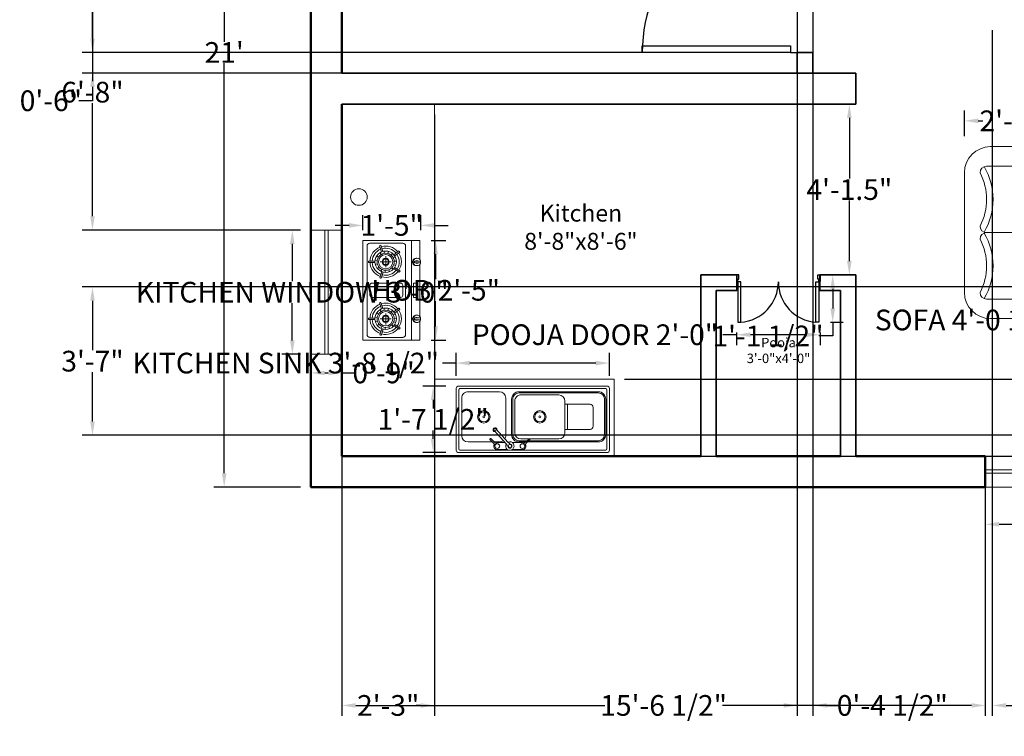
# Model space of a CAD drawing. Units: inches. Extents: x -59 to 502, y -260 to 136.
# Tile 1 of 8: x -59 to 226, y -260 to -53. Entities that reach past the tile are written whole.
import ezdxf

# ---------------------------------------------------------------- set-up
doc = ezdxf.new("R2010")
doc.units = ezdxf.units.IN
doc.header["$MEASUREMENT"] = 0
for name, color, linetype, lineweight in [('A-ANNO-DIMS', 2, 'Continuous', 18), ('A-AREA-IDEN', 7, 'Continuous', 25), ('A-FLOR-CASE', 9, 'Continuous', 18), ('Doors', 18, 'Continuous', 25), ('Inner wall', 11, 'Continuous', 35), ('Kitchen Appliances', 80, 'Continuous', 18), ('Outer Wall', 10, 'Continuous', 50), ('Sink', 62, 'Continuous', 18), ('Sofas', 84, 'Continuous', 18), ('Windows', 150, 'Continuous', 18)]:
    doc.layers.add(name, color=color, linetype=linetype, lineweight=lineweight)
doc.styles.get("Standard").update_dxf_attribs({"font": 'arial.ttf'})
doc.dimstyles.get("Standard").update_dxf_attribs({"dimtxt": 6, "dimasz": 4, "dimexe": 3, "dimexo": 3, "dimgap": 0.09, "dimtad": 0, "dimtih": 1, "dimtoh": 1, "dimdec": 1, "dimzin": 0, "dimdsep": 46, "dimlunit": 3, "dimtxsty": 'Standard', "dimcen": 0.09, "dimadec": 0, "dimazin": 0, "dimtfac": 1, "dimtdec": 1, "dimtofl": 0, "dimtmove": 0, "dimatfit": 3, "dimfxl": 1, "dimtolj": 1, "dimtzin": 0, "dimarcsym": 0})

# ---------------------------------------------------------------- blocks, each defined once
blk = doc.blocks.new('Window')
for p, q in [((868.39, 234.72), (940.39, 234.72)), ((868.39, 225.72), (868.39, 234.72)), ((940.39, 234.72), (940.39, 225.72)), ((868.39, 230.72), (940.39, 230.72)), ((940.39, 229.72), (868.39, 229.72)), ((940.39, 225.72), (868.39, 225.72))]:
    blk.add_line(p, q)
blk = doc.blocks.new('*D6')
at = {"layer": 'A-ANNO-DIMS', "color": 0, "lineweight": -2, "transparency": 16777216}
for p, q in [((22.46, 63.92), (-2.69, 63.92)), ((0.31, 59.92), (0.31, -58.98)), ((0.31, -184.08), (0.31, -65.18)), ((22.46, -188.08), (-2.69, -188.08))]:
    blk.add_line(p, q, dxfattribs=at)
at = {"layer": 'A-ANNO-DIMS', "color": 0, "transparency": 16777216}
for points in [[(-0.35, 59.92), (0.98, 59.92), (0.31, 63.92)], [(-0.35, -184.08), (0.98, -184.08), (0.31, -188.08)]]:
    blk.add_solid(points, dxfattribs=at)
at = {"layer": 'Defpoints', "color": 0, "transparency": 16777216}
for p in [(25.46, 63.92), (0.31, -188.08), (25.46, -188.08)]:
    blk.add_point(p, dxfattribs=at)
at = {"layer": 'A-ANNO-DIMS', "color": 0, "transparency": 16777216, "insert": (0.31, -62.08), "char_height": 6, "attachment_point": 5}
blk.add_mtext("\\A1;21'", dxfattribs=at)
blk = doc.blocks.new('*U11')
for p, q in [((-40, 0), (-40, 6)), ((0, 0), (0, 6))]:
    blk.add_line(p, q)
blk.add_lwpolyline([(0, 0), (0, -40), (-1.75, -40), (-1.75, 0)], close=True)
blk.add_arc((0, 0), 40, 180, 270)
blk = doc.blocks.new('Kitchen Window KW')
for p, q in [((875.78, 183.9), (911.78, 183.9)), ((875.78, 174.9), (875.78, 183.9)), ((911.78, 183.9), (911.78, 174.9)), ((875.78, 179.9), (911.78, 179.9)), ((911.78, 178.9), (875.78, 178.9)), ((911.78, 174.9), (875.78, 174.9))]:
    blk.add_line(p, q)
blk = doc.blocks.new('A$C16D51D41')
for p, q in [((1.12, 0.69, -343.199), (0.2, 0.69, -343.199)), ((0, 0.49, -343.199), (0, 0.06, -343.199)), ((0.15, 0.52, -343.199), (0.15, 0.06, -343.199)), ((0.15, 0.06, -343.199), (0.15, 0.52, -343.199)), ((0.15, 0.52, -343.199), (0.15, 0.06, -343.199)), ((0.66, 0.06, -343.199), (0.66, 0.52, -343.199)), ((0.66, 0.52, -343.199), (0.66, 0.06, -343.199)), ((1.17, 0.52, -343.199), (1.17, 0.06, -343.199)), ((1.32, 0.06, -343.199), (1.32, 0.49, -343.199)), ((0, 0.06, -343.199), (0.15, 0.06, -343.199)), ((1.32, 0.06, -343.199), (1.17, 0.06, -343.199))]:
    blk.add_line(p, q)
for centre, radius, start, end in [((0.2, 0.49, -343.199), 0.2, 90, 180), ((1.12, 0.49, -343.199), 0.2, 0, 90), ((0.2, 0.52, -343.199), 0.05, 90, 180), ((0.405, 0.9652, -343.199), 0.4953, 239.49109, 300.50891), ((0.405, 0.9652, -343.199), 0.4453, 242.58608, 297.41392), ((0.61, 0.52, -343.199), 0.05, 0, 90), ((0.71, 0.52, -343.199), 0.05, 90, 180), ((0.915, 0.9652, -343.199), 0.4953, 239.49109, 300.50891), ((0.915, 0.9652, -343.199), 0.4453, 242.58608, 297.41392), ((1.12, 0.52, -343.199), 0.05, 0, 90), ((0.405, 0.5719, -343.199), 0.5719, 243.51896, 296.48104), ((0.915, 0.5719, -343.199), 0.5719, 243.51896, 296.48104)]:
    blk.add_arc(centre, radius, start, end)
blk = doc.blocks.new('A$C5D256BD7')
for points in [[(60, 678), (60, 100), (20, 100), (20, 678)], [(1140, 678), (1140, 100), (1180, 100), (1180, 678)], [(6, 10), (0, 10), (0, 90), (6, 90)], [(6, 100), (20, 100), (20, 60), (32, 60), (32, 16), (32, 0), (6, 0)], [(1194, 100), (1180, 100), (1180, 60), (1168, 60), (1168, 16), (1168, 0), (1194, 0)], [(1194, 10), (1200, 10), (1200, 90), (1194, 90)]]:
    blk.add_lwpolyline(points, close=True)
for centre, start, end in [((21, 100), 359.9362, 86.0902), ((1179, 100), 93.9098, 180.0638)]:
    blk.add_arc(centre, 579, start, end)
blk = doc.blocks.new('Kitchen Sink Set')
at = {"color": 0}
for p, q in [((1319.2, 504.5), (1319.2, 30.2)), ((2480.8, 523.9), (1338.6, 523.9)), ((1338.6, 494.8), (1338.6, 39.9)), ((2078, 504.5), (1348.2, 504.5)), ((2068.2, 500.1), (1989.5, 500.1)), ((2471.1, 504.5), (2094.7, 504.5)), ((2183.1, 500.1), (2104.5, 500.1)), ((2112.8, 458.4), (2208, 354)), ((2480.8, 39.9), (2480.8, 494.8)), ((2500.2, 504.5), (2500.2, 30.2)), ((1347.4, 383.5), (1347.4, 112.5)), ((1356.3, 383.5), (1356.3, 112.5)), ((1950.6, 441.6), (1405.5, 441.6)), ((1941.6, 432.7), (1405.5, 432.7)), ((1710.4, 417.4), (1933.2, 417.4)), ((1957.7, 448.5), (1934.5, 425.7)), ((1940.2, 417.4), (2000.8, 417.4)), ((1964.5, 441.6), (1941.3, 418.8)), ((2015.4, 432.7), (1955.4, 432.7)), ((2015.4, 441.6), (1964.4, 441.6)), ((2068.2, 446), (1989.5, 446)), ((2063.8, 112.5), (2063.8, 383.5)), ((2073.4, 112.5), (2073.4, 383.5)), ((2098.5, 445.3), (2193.7, 340.9)), ((2117.8, 102.8), (2117.8, 393.2)), ((2183.1, 446), (2124.1, 446)), ((2166.2, 441.6), (2207.3, 441.6)), ((2207.7, 441.2), (2230.5, 418)), ((2214.6, 448), (2237.4, 424.8)), ((2220.8, 441.6), (2408.2, 441.6)), ((2456.6, 102.8), (2456.6, 393.2)), ((1444.2, 320.6), (1444.2, 175.4)), ((1662, 344.8), (1468.4, 344.8)), ((1642.7, 151.2), (1642.7, 344.8)), ((1662, 127), (1662, 369)), ((2049.2, 127), (2049.2, 369)), ((1662, 151.2), (1468.4, 151.2)), ((1710.4, 78.6), (2000.8, 78.6)), ((1338.6, 10.8), (2480.8, 10.8)), ((1348.2, 30.2), (2471.1, 30.2)), ((1405.5, 64.1), (2015.4, 64.1)), ((1405.5, 54.4), (2015.4, 54.4)), ((2166.2, 54.4), (2408.2, 54.4))]:
    blk.add_line(p, q, dxfattribs=at)
for centre, radius in [((1989.5, 473), 18.1), ((2086.3, 473), 12.4), ((2183.1, 473), 18.1), ((2201.5, 346.7), 9.73), ((1855.6, 248), 48.4), ((1855.6, 248), 38.7), ((1855.6, 248), 8.23), ((2287.2, 248), 48.4), ((2287.2, 248), 38.7), ((2287.2, 248), 8.23)]:
    blk.add_circle(centre, radius, dxfattribs=at)
for centre, radius, start, end in [((1338.6, 504.5), 19.4, 90, 180), ((1348.2, 494.8), 9.68, 90, 180), ((1923.8, 483.1), 48.4, 314.49562, 351.33895), ((1989.5, 473), 27, 90, 209.88157), ((2086.3, 473), 32.5, 329.64442, 295.0423), ((2086.3, 473), 16.4, 16.07549, 248.61123), ((2062.7, 412.7), 48.4, 42.34336, 68.61123), ((2148.6, 491), 48.4, 196.07549, 222.34336), ((2183.1, 473), 27, 329.10967, 90), ((2249.1, 481.9), 48.4, 187.65229, 224.49562), ((2471.1, 494.8), 9.68, 0, 90), ((2480.8, 504.5), 19.4, 0, 90), ((1405.5, 383.5), 58.1, 90, 180), ((1405.5, 383.5), 49.2, 90, 180), ((1710.4, 369), 48.4, 90, 180), ((1710.4, 369), 48.4, 90, 91.14555), ((1936.7, 421.1), 5.11, 115.72387, 333.26737), ((1998.4, 407.1), 48.4, 97.65229, 134.49562), ((1989.5, 473), 27, 239.10967, 270), ((2000.8, 369), 48.4, 0, 90), ((2015.4, 383.5), 58.1, 0, 90), ((2013.9, 382.9), 49.8, 0.67291, 88.37528), ((2166.2, 393.2), 48.4, 150.29154, 180), ((2166.2, 393.2), 48.4, 90, 127.0737), ((2173.1, 407.3), 48.4, 44.49562, 81.33895), ((2183.1, 473), 27, 270, 299.88157), ((2235.1, 420.2), 5.11, 205.72387, 63.26737), ((2408.2, 393.2), 48.4, 0, 90), ((1468.4, 320.6), 24.2, 90, 180), ((2200.8, 347.4), 15.7, 170.3658, 94.32092), ((1468.4, 175.4), 24.2, 180, 270), ((1405.5, 112.5), 58.1, 180, 270), ((1406.1, 113.9), 49.8, 181.62472, 269.32709), ((1710.4, 127), 48.4, 180, 270), ((2000.8, 127), 48.4, 270, 0), ((2015.4, 112.5), 58.1, 270, 0), ((2015.4, 112.5), 48.4, 270, 0), ((2166.2, 102.8), 48.4, 180, 270), ((2408.2, 102.8), 48.4, 270, 0), ((1338.6, 30.2), 19.4, 180, 270), ((1348.2, 39.9), 9.68, 180, 270), ((2471.1, 39.9), 9.68, 270, 0), ((2480.8, 30.2), 19.4, 270, 0)]:
    blk.add_arc(centre, radius, start, end, dxfattribs=at)
blk = doc.blocks.new('Gas Stove')
for p, q in [((1373.89, 868.55), (1373.89, 856.72)), ((1373.89, 868.55), (1394.6, 868.55)), ((1375.08, 867.67), (1393.41, 867.67)), ((1394.6, 868.55), (1394.6, 856.72)), ((1374.48, 867.08), (1374.48, 860.27)), ((1377.75, 865.97), (1377.87, 865.54)), ((1378.18, 866.04), (1378.18, 867.37)), ((1378.48, 866.04), (1378.48, 867.37)), ((1378.68, 866.01), (1378.61, 865.58)), ((1379.54, 865.68), (1379.3, 865.31)), ((1382.77, 866.63), (1382.77, 860.72)), ((1383.21, 867.08), (1385.28, 867.08)), ((1385.72, 866.63), (1385.72, 860.72)), ((1389.59, 865.97), (1389.7, 865.54)), ((1390.01, 866.04), (1390.01, 867.37)), ((1390.31, 866.04), (1390.31, 867.37)), ((1390.51, 866.01), (1390.44, 865.58)), ((1391.37, 865.68), (1391.13, 865.31)), ((1394, 867.08), (1394, 860.27)), ((1374.9, 864.75), (1376.17, 864.35)), ((1374.99, 865.03), (1376.26, 864.63)), ((1376.11, 863.94), (1376.56, 863.92)), ((1376.35, 864.83), (1376.75, 864.63)), ((1376.93, 865.55), (1377.21, 865.2)), ((1377.16, 863.82), (1379.45, 863.82)), ((1378.33, 864.99), (1378.33, 862.65)), ((1380.19, 865.03), (1379.82, 864.79)), ((1380.52, 864.17), (1380.08, 864.1)), ((1381.65, 865.09), (1380.38, 864.66)), ((1381.74, 864.81), (1380.48, 864.38)), ((1386.73, 864.75), (1388, 864.35)), ((1386.82, 865.03), (1388.09, 864.63)), ((1387.94, 863.94), (1388.39, 863.92)), ((1388.18, 864.83), (1388.58, 864.63)), ((1388.76, 865.55), (1389.04, 865.2)), ((1389.01, 863.82), (1391.31, 863.82)), ((1390.16, 864.99), (1390.16, 862.65)), ((1392.02, 865.03), (1391.65, 864.79)), ((1392.35, 864.17), (1391.91, 864.1)), ((1393.48, 865.09), (1392.21, 864.66)), ((1393.57, 864.81), (1392.31, 864.38)), ((1376.15, 861.02), (1376.92, 862.11)), ((1376.26, 863.03), (1376.67, 863.19)), ((1376.39, 860.85), (1377.16, 861.94)), ((1376.76, 862.25), (1377.07, 862.57)), ((1377.53, 861.75), (1377.69, 862.17)), ((1378.44, 861.61), (1378.42, 862.05)), ((1379.34, 861.85), (1379.13, 862.24)), ((1380.32, 860.88), (1379.53, 861.95)), ((1380.05, 862.43), (1379.71, 862.71)), ((1380.56, 861.06), (1379.76, 862.13)), ((1380.47, 863.25), (1380.04, 863.36)), ((1387.98, 861.02), (1388.75, 862.11)), ((1388.09, 863.03), (1388.5, 863.19)), ((1388.22, 860.85), (1388.99, 861.94)), ((1388.59, 862.25), (1388.9, 862.57)), ((1389.36, 861.75), (1389.52, 862.17)), ((1390.28, 861.61), (1390.25, 862.05)), ((1391.17, 861.85), (1390.97, 862.24)), ((1392.15, 860.88), (1391.36, 861.95)), ((1391.88, 862.43), (1391.54, 862.71)), ((1392.39, 861.06), (1391.59, 862.13)), ((1392.3, 863.25), (1391.87, 863.36)), ((1375.08, 859.68), (1393.41, 859.68)), ((1383.21, 860.27), (1385.28, 860.27)), ((1373.89, 858.5), (1394.6, 858.5)), ((1378.15, 857.84), (1378.51, 857.84)), ((1378.15, 857.84), (1378.15, 856.59)), ((1378.51, 857.84), (1378.51, 856.59)), ((1382.77, 858.07), (1382.77, 857.18)), ((1382.77, 858.07), (1385.72, 858.07)), ((1385.72, 858.07), (1385.72, 857.18)), ((1389.94, 857.84), (1390.29, 857.84)), ((1389.94, 857.84), (1389.94, 856.59)), ((1390.29, 857.84), (1390.29, 856.59)), ((1373.89, 856.72), (1377.86, 856.72)), ((1378.79, 856.72), (1389.65, 856.72)), ((1382.77, 857.18), (1385.72, 857.18)), ((1390.57, 856.72), (1394.6, 856.72))]:
    blk.add_line(p, q)
for centre, radius in [((1378.33, 863.82), 2.22), ((1390.16, 863.82), 2.22), ((1378.33, 863.82), 1.77), ((1378.33, 863.82), 1.48), ((1378.33, 863.82), 0.739), ((1378.33, 863.82), 0.592), ((1390.16, 863.82), 1.77), ((1390.16, 863.82), 1.48), ((1390.16, 863.82), 0.739), ((1390.16, 863.82), 0.592)]:
    blk.add_circle(centre, radius)
for centre, radius, start, end in [((1375.08, 867.08), 0.592, 90, 180), ((1393.41, 867.08), 0.592, 0, 90), ((1378.33, 863.82), 3.25, 92.6053, 159.852), ((1378.33, 863.82), 2.81, 93.017, 159.4403), ((1378.33, 863.82), 3.55, 87.612, 92.388), ((1378.33, 863.82), 3.25, 21.0625, 87.3947), ((1378.33, 863.82), 2.81, 21.4742, 86.983), ((1383.21, 866.63), 0.444, 90, 180), ((1385.28, 866.63), 0.444, 0, 90), ((1390.16, 863.82), 3.25, 92.6053, 159.852), ((1390.16, 863.82), 2.81, 93.017, 159.4403), ((1390.16, 863.82), 3.55, 87.612, 92.388), ((1390.16, 863.82), 3.25, 21.0625, 87.3947), ((1390.16, 863.82), 2.81, 21.4742, 86.983), ((1378.33, 863.82), 3.55, 160.0692, 164.8452), ((1378.33, 863.82), 3.25, 165.0625, 231.852), ((1378.33, 863.82), 2.81, 165.4742, 231.4403), ((1378.33, 863.82), 2.81, 309.4742, 15.4403), ((1378.33, 863.82), 3.25, 309.0625, 15.852), ((1378.33, 863.82), 3.55, 16.0692, 20.8452), ((1390.16, 863.82), 3.55, 160.0692, 164.8452), ((1390.16, 863.82), 3.25, 165.0625, 231.852), ((1390.16, 863.82), 2.81, 165.4742, 231.4403), ((1390.16, 863.82), 2.81, 309.4742, 15.4403), ((1390.16, 863.82), 3.25, 309.0625, 15.852), ((1390.16, 863.82), 3.55, 16.0692, 20.8452), ((1375.08, 860.27), 0.592, 180, 270), ((1378.33, 863.82), 3.55, 232.0692, 236.8452), ((1378.33, 863.82), 3.25, 237.0625, 303.852), ((1378.33, 863.82), 2.81, 237.4742, 303.4403), ((1378.33, 863.82), 3.55, 304.0692, 308.8452), ((1383.21, 860.72), 0.444, 180, 270), ((1385.28, 860.72), 0.444, 270, 0), ((1390.16, 863.82), 3.55, 232.0692, 236.8452), ((1390.16, 863.82), 3.25, 237.0625, 303.852), ((1390.16, 863.82), 2.81, 237.4742, 303.4403), ((1390.16, 863.82), 3.55, 304.0692, 308.8452), ((1393.41, 860.27), 0.592, 270, 0), ((1378.32, 857.51), 0.76, 157.5, 180), ((1378.32, 857.33), 0.76, 157.5, 180), ((1378.32, 857.51), 0.76, 180, 187.0423), ((1378.32, 857.51), 0.76, 135, 157.5), ((1378.32, 857.33), 0.76, 135, 157.5), ((1378.32, 857.51), 0.76, 112.5, 135), ((1378.32, 857.33), 0.76, 112.5, 135), ((1378.32, 857.51), 0.76, 90, 112.5), ((1378.32, 857.33), 0.76, 90, 112.5), ((1378.32, 857.38), 0.288, 124.9148, 235.0852), ((1378.32, 857.51), 0.76, 67.5, 90), ((1378.32, 857.33), 0.76, 67.5, 90), ((1378.32, 857.38), 0.288, 311.223, 48.777), ((1378.32, 857.51), 0.76, 45, 67.5), ((1378.32, 857.33), 0.76, 45, 67.5), ((1378.32, 857.51), 0.76, 22.5, 45), ((1378.32, 857.33), 0.76, 22.5, 45), ((1378.32, 857.51), 0.76, 0, 22.5), ((1378.32, 857.33), 0.76, 0, 22.5), ((1378.32, 857.51), 0.76, 352.9577, 0), ((1390.11, 857.51), 0.76, 157.5, 180), ((1390.11, 857.33), 0.76, 157.5, 180), ((1390.11, 857.51), 0.76, 180, 187.0423), ((1390.11, 857.51), 0.76, 135, 157.5), ((1390.11, 857.33), 0.76, 135, 157.5), ((1390.11, 857.51), 0.76, 112.5, 135), ((1390.11, 857.33), 0.76, 112.5, 135), ((1390.11, 857.51), 0.76, 90, 112.5), ((1390.11, 857.33), 0.76, 90, 112.5), ((1390.1, 857.38), 0.288, 124.9148, 235.0852), ((1390.11, 857.51), 0.76, 67.5, 90), ((1390.11, 857.33), 0.76, 67.5, 90), ((1390.1, 857.38), 0.288, 311.223, 48.777), ((1390.11, 857.51), 0.76, 45, 67.5), ((1390.11, 857.33), 0.76, 45, 67.5), ((1390.11, 857.51), 0.76, 22.5, 45), ((1390.11, 857.33), 0.76, 22.5, 45), ((1390.11, 857.51), 0.76, 0, 22.5), ((1390.11, 857.33), 0.76, 0, 22.5), ((1390.11, 857.51), 0.76, 352.9577, 0), ((1378.32, 857.33), 0.76, 180, 202.5), ((1378.32, 857.33), 0.76, 202.5, 225), ((1378.32, 857.33), 0.76, 225, 247.5), ((1378.32, 857.33), 0.76, 247.5, 270), ((1378.32, 857.33), 0.76, 270, 292.5), ((1378.32, 857.33), 0.76, 292.5, 315), ((1378.32, 857.33), 0.76, 315, 337.5), ((1378.32, 857.33), 0.76, 337.5, 0), ((1390.11, 857.33), 0.76, 180, 202.5), ((1390.11, 857.33), 0.76, 202.5, 225), ((1390.11, 857.33), 0.76, 225, 247.5), ((1390.11, 857.33), 0.76, 247.5, 270), ((1390.11, 857.33), 0.76, 270, 292.5), ((1390.11, 857.33), 0.76, 292.5, 315), ((1390.11, 857.33), 0.76, 315, 337.5), ((1390.11, 857.33), 0.76, 337.5, 0)]:
    blk.add_arc(centre, radius, start, end)
blk = doc.blocks.new('*D22')
at = {"layer": 'A-ANNO-DIMS', "color": 0, "lineweight": -2, "transparency": 16777216}
for p, q in [((180.46, -77.08), (178.54, -77.08)), ((181.54, -81.08), (181.54, -98.67)), ((181.54, -122.58), (181.54, -104.98)), ((180.46, -126.58), (178.54, -126.58))]:
    blk.add_line(p, q, dxfattribs=at)
at = {"layer": 'A-ANNO-DIMS', "color": 0, "transparency": 16777216}
for points in [[(180.87, -81.08), (182.2, -81.08), (181.54, -77.08)], [(180.87, -122.58), (182.2, -122.58), (181.54, -126.58)]]:
    blk.add_solid(points, dxfattribs=at)
at = {"layer": 'Defpoints', "color": 0, "transparency": 16777216}
for p in [(183.46, -77.08), (181.54, -126.58), (183.46, -126.58)]:
    blk.add_point(p, dxfattribs=at)
at = {"layer": 'A-ANNO-DIMS', "color": 0, "transparency": 16777216, "insert": (181.54, -101.83), "char_height": 6, "attachment_point": 5}
blk.add_mtext('\\A1;4\'-1.5"', dxfattribs=at)
blk = doc.blocks.new('*D25')
at = {"layer": 'A-ANNO-DIMS', "color": 0, "lineweight": -2, "transparency": 16777216}
for p, q in [((247.8, -143.9), (247.8, -136.64)), ((296.18, -143.9), (296.18, -136.64)), ((247.8, -139.64), (243.8, -139.64)), ((292.18, -139.64), (251.8, -139.64))]:
    blk.add_line(p, q, dxfattribs=at)
at = {"layer": 'A-ANNO-DIMS', "color": 0, "transparency": 16777216}
for points in [[(251.8, -138.97), (251.8, -140.31), (247.8, -139.64)], [(292.18, -138.97), (292.18, -140.31), (296.18, -139.64)]]:
    blk.add_solid(points, dxfattribs=at)
at = {"layer": 'Defpoints', "color": 0, "transparency": 16777216}
for p in [(247.8, -139.64), (247.8, -146.9), (296.18, -146.9)]:
    blk.add_point(p, dxfattribs=at)
at = {"layer": 'A-ANNO-DIMS', "color": 0, "transparency": 16777216, "insert": (216.18, -139.64), "char_height": 6, "attachment_point": 5}
blk.add_mtext('\\A1;SOFA 4\'-0 1/2"', dxfattribs=at)
blk = doc.blocks.new('*D28')
at = {"layer": 'A-ANNO-DIMS', "color": 0, "lineweight": -2, "transparency": 16777216}
for p, q in [((214.91, -86.38), (214.91, -78.9)), ((241.73, -86.38), (241.73, -78.9)), ((218.91, -81.9), (220.2, -81.9)), ((237.73, -81.9), (236.43, -81.9))]:
    blk.add_line(p, q, dxfattribs=at)
at = {"layer": 'A-ANNO-DIMS', "color": 0, "transparency": 16777216}
for points in [[(218.91, -81.24), (218.91, -82.57), (214.91, -81.9)], [(237.73, -81.24), (237.73, -82.57), (241.73, -81.9)]]:
    blk.add_solid(points, dxfattribs=at)
at = {"layer": 'Defpoints', "color": 0, "transparency": 16777216}
for p in [(214.91, -81.9), (214.91, -89.38), (241.73, -89.38)]:
    blk.add_point(p, dxfattribs=at)
at = {"layer": 'A-ANNO-DIMS', "color": 0, "transparency": 16777216, "insert": (228.32, -81.9), "char_height": 6, "attachment_point": 5}
blk.add_mtext('\\A1;2\'-3"', dxfattribs=at)
blk = doc.blocks.new('*D37')
at = {"layer": 'A-ANNO-DIMS', "color": 0, "lineweight": -2, "transparency": 16777216}
for p, q in [((220.96, -191.08), (220.96, -201.88)), ((292.96, -191.08), (292.96, -201.88)), ((224.96, -198.88), (229.22, -198.88)), ((288.96, -198.88), (284.7, -198.88))]:
    blk.add_line(p, q, dxfattribs=at)
at = {"layer": 'A-ANNO-DIMS', "color": 0, "transparency": 16777216}
for points in [[(224.96, -198.21), (224.96, -199.54), (220.96, -198.88)], [(288.96, -198.21), (288.96, -199.54), (292.96, -198.88)]]:
    blk.add_solid(points, dxfattribs=at)
at = {"layer": 'Defpoints', "color": 0, "transparency": 16777216}
for p in [(220.96, -188.08), (292.96, -188.08), (292.96, -198.88)]:
    blk.add_point(p, dxfattribs=at)
at = {"layer": 'A-ANNO-DIMS', "color": 0, "transparency": 16777216, "insert": (256.96, -198.88), "char_height": 6, "attachment_point": 5}
blk.add_mtext('\\A1;WINDOW 6\'-0"', dxfattribs=at)
blk = doc.blocks.new('*D43')
at = {"layer": 'A-ANNO-DIMS', "color": 0, "lineweight": -2, "transparency": 16777216}
for p, q in [((22.46, -113.59), (17.06, -113.59)), ((20.06, -117.59), (20.06, -128.4)), ((20.06, -145.59), (20.06, -134.79)), ((22.46, -149.59), (17.06, -149.59))]:
    blk.add_line(p, q, dxfattribs=at)
at = {"layer": 'A-ANNO-DIMS', "color": 0, "transparency": 16777216}
for points in [[(19.39, -117.59), (20.73, -117.59), (20.06, -113.59)], [(19.39, -145.59), (20.73, -145.59), (20.06, -149.59)]]:
    blk.add_solid(points, dxfattribs=at)
at = {"layer": 'Defpoints', "color": 0, "transparency": 16777216}
for p in [(25.46, -113.59), (20.06, -149.59), (25.46, -149.59)]:
    blk.add_point(p, dxfattribs=at)
at = {"layer": 'A-ANNO-DIMS', "color": 0, "transparency": 16777216, "insert": (20.06, -131.59), "char_height": 6, "attachment_point": 5}
blk.add_mtext('\\A1;KITCHEN WINDOW 3\'-0"', dxfattribs=at)
blk = doc.blocks.new('*D44')
at = {"layer": 'A-ANNO-DIMS', "color": 0, "lineweight": -2, "transparency": 16777216}
for p, q in [((25.46, -152.59), (25.46, -157.99)), ((34.46, -152.59), (34.46, -157.99)), ((29.46, -154.99), (30.46, -154.99)), ((34.46, -154.99), (38.46, -154.99))]:
    blk.add_line(p, q, dxfattribs=at)
at = {"layer": 'A-ANNO-DIMS', "color": 0, "transparency": 16777216}
for points in [[(29.46, -154.33), (29.46, -155.66), (25.46, -154.99)], [(30.46, -154.33), (30.46, -155.66), (34.46, -154.99)]]:
    blk.add_solid(points, dxfattribs=at)
at = {"layer": 'Defpoints', "color": 0, "transparency": 16777216}
for p in [(25.46, -149.59), (34.46, -149.59), (34.46, -154.99)]:
    blk.add_point(p, dxfattribs=at)
at = {"layer": 'A-ANNO-DIMS', "color": 0, "transparency": 16777216, "insert": (46.52, -154.99), "char_height": 6, "attachment_point": 5}
blk.add_mtext('\\A1;0\'-9"', dxfattribs=at)
blk = doc.blocks.new('*D49')
at = {"layer": 'A-ANNO-DIMS', "color": 0, "lineweight": -2, "transparency": 16777216}
for p, q in [((148.84, -143.92), (144.84, -143.92)), ((148.84, -143.28), (148.84, -146.92)), ((169.08, -143.92), (152.84, -143.92)), ((173.08, -143.28), (173.08, -146.92))]:
    blk.add_line(p, q, dxfattribs=at)
at = {"layer": 'A-ANNO-DIMS', "color": 0, "transparency": 16777216}
for points in [[(152.84, -143.25), (152.84, -144.58), (148.84, -143.92)], [(169.08, -143.25), (169.08, -144.58), (173.08, -143.92)]]:
    blk.add_solid(points, dxfattribs=at)
at = {"layer": 'Defpoints', "color": 0, "transparency": 16777216}
for p in [(148.84, -140.28), (173.08, -140.28), (148.84, -143.92)]:
    blk.add_point(p, dxfattribs=at)
at = {"layer": 'A-ANNO-DIMS', "color": 0, "transparency": 16777216, "insert": (107.81, -143.92), "char_height": 6, "attachment_point": 5}
blk.add_mtext('\\A1;POOJA DOOR 2\'-0"', dxfattribs=at)
blk = doc.blocks.new('*D50')
at = {"layer": 'A-ANNO-DIMS', "color": 0, "lineweight": -2, "transparency": 16777216}
for p, q in [((176.08, -126.58), (179.72, -126.58)), ((176.72, -130.58), (176.72, -136.28)), ((176.08, -140.28), (179.72, -140.28)), ((176.72, -140.28), (176.72, -144.28)), ((176.72, -144.28), (172.72, -144.28))]:
    blk.add_line(p, q, dxfattribs=at)
at = {"layer": 'A-ANNO-DIMS', "color": 0, "transparency": 16777216}
for points in [[(176.05, -130.58), (177.39, -130.58), (176.72, -126.58)], [(176.05, -136.28), (177.39, -136.28), (176.72, -140.28)]]:
    blk.add_solid(points, dxfattribs=at)
at = {"layer": 'Defpoints', "color": 0, "transparency": 16777216}
for p in [(173.08, -126.58), (173.08, -140.28), (176.72, -140.28)]:
    blk.add_point(p, dxfattribs=at)
at = {"layer": 'A-ANNO-DIMS', "color": 0, "transparency": 16777216, "insert": (157.95, -144.28), "char_height": 6, "attachment_point": 5}
blk.add_mtext('\\A1;1\'-1 1/2"', dxfattribs=at)
blk = doc.blocks.new('*D51')
at = {"layer": 'A-ANNO-DIMS', "color": 0, "lineweight": -2, "transparency": 16777216}
for p, q in [((67.56, -155.81), (67.56, -149.14)), ((112, -155.81), (112, -149.14)), ((67.56, -152.14), (63.56, -152.14)), ((108, -152.14), (71.56, -152.14))]:
    blk.add_line(p, q, dxfattribs=at)
at = {"layer": 'A-ANNO-DIMS', "color": 0, "transparency": 16777216}
for points in [[(71.56, -151.48), (71.56, -152.81), (67.56, -152.14)], [(108, -151.48), (108, -152.81), (112, -152.14)]]:
    blk.add_solid(points, dxfattribs=at)
at = {"layer": 'Defpoints', "color": 0, "transparency": 16777216}
for p in [(67.56, -152.14), (67.56, -158.81), (112, -158.81)]:
    blk.add_point(p, dxfattribs=at)
at = {"layer": 'A-ANNO-DIMS', "color": 0, "transparency": 16777216, "insert": (18.14, -152.14), "char_height": 6, "attachment_point": 5}
blk.add_mtext('\\A1;KITCHEN SINK 3\'-8 1/2"', dxfattribs=at)
blk = doc.blocks.new('*D52')
at = {"layer": 'A-ANNO-DIMS', "color": 0, "lineweight": -2, "transparency": 16777216}
for p, q in [((64.56, -158.81), (57.9, -158.81)), ((60.9, -162.81), (60.9, -165.27)), ((60.9, -174.11), (60.9, -171.65)), ((64.56, -178.11), (57.9, -178.11))]:
    blk.add_line(p, q, dxfattribs=at)
at = {"layer": 'A-ANNO-DIMS', "color": 0, "transparency": 16777216}
for points in [[(60.23, -162.81), (61.56, -162.81), (60.9, -158.81)], [(60.23, -174.11), (61.56, -174.11), (60.9, -178.11)]]:
    blk.add_solid(points, dxfattribs=at)
at = {"layer": 'Defpoints', "color": 0, "transparency": 16777216}
for p in [(67.56, -158.81), (60.9, -178.11), (67.56, -178.11)]:
    blk.add_point(p, dxfattribs=at)
at = {"layer": 'A-ANNO-DIMS', "color": 0, "transparency": 16777216, "insert": (60.9, -168.46), "char_height": 6, "attachment_point": 5}
blk.add_mtext('\\A1;1\'-7 1/2"', dxfattribs=at)
blk = doc.blocks.new('*D53')
at = {"layer": 'A-ANNO-DIMS', "color": 0, "lineweight": -2, "transparency": 16777216}
for p, q in [((60.27, -116.56), (64.61, -116.56)), ((61.61, -120.56), (61.61, -127.84)), ((61.61, -141.51), (61.61, -134.23)), ((60.27, -145.51), (64.61, -145.51))]:
    blk.add_line(p, q, dxfattribs=at)
at = {"layer": 'A-ANNO-DIMS', "color": 0, "transparency": 16777216}
for points in [[(60.95, -120.56), (62.28, -120.56), (61.61, -116.56)], [(60.95, -141.51), (62.28, -141.51), (61.61, -145.51)]]:
    blk.add_solid(points, dxfattribs=at)
at = {"layer": 'Defpoints', "color": 0, "transparency": 16777216}
for p in [(57.27, -116.56), (61.61, -116.56), (57.27, -145.51)]:
    blk.add_point(p, dxfattribs=at)
at = {"layer": 'A-ANNO-DIMS', "color": 0, "transparency": 16777216, "insert": (61.61, -131.03), "char_height": 6, "attachment_point": 5}
blk.add_mtext('\\A1;HOB 2\'-5"', dxfattribs=at)
blk = doc.blocks.new('*D54')
at = {"layer": 'A-ANNO-DIMS', "color": 0, "lineweight": -2, "transparency": 16777216}
for p, q in [((40.51, -113.56), (40.51, -109.22)), ((57.27, -113.56), (57.27, -109.22)), ((36.51, -112.22), (32.51, -112.22)), ((61.27, -112.22), (65.27, -112.22))]:
    blk.add_line(p, q, dxfattribs=at)
at = {"layer": 'A-ANNO-DIMS', "color": 0, "transparency": 16777216}
for points in [[(36.51, -111.55), (36.51, -112.89), (40.51, -112.22)], [(61.27, -111.55), (61.27, -112.89), (57.27, -112.22)]]:
    blk.add_solid(points, dxfattribs=at)
at = {"layer": 'Defpoints', "color": 0, "transparency": 16777216}
for p in [(40.51, -112.22), (40.51, -116.56), (57.27, -116.56)]:
    blk.add_point(p, dxfattribs=at)
at = {"layer": 'A-ANNO-DIMS', "color": 0, "transparency": 16777216, "insert": (48.89, -112.22), "char_height": 6, "attachment_point": 5}
blk.add_mtext('\\A1;1\'-5"', dxfattribs=at)
blk = doc.blocks.new('*D60')
at = {"layer": 'A-ANNO-DIMS', "color": 0, "lineweight": -2, "transparency": 16777216}
for p, q in [((22.46, -33.59), (-40.87, -33.59)), ((-37.87, -37.59), (-37.87, -70.44)), ((-37.87, -109.59), (-37.87, -76.75)), ((22.46, -113.59), (-40.87, -113.59))]:
    blk.add_line(p, q, dxfattribs=at)
at = {"layer": 'A-ANNO-DIMS', "color": 0, "transparency": 16777216}
for points in [[(-38.53, -37.59), (-37.2, -37.59), (-37.87, -33.59)], [(-38.53, -109.59), (-37.2, -109.59), (-37.87, -113.59)]]:
    blk.add_solid(points, dxfattribs=at)
at = {"layer": 'Defpoints', "color": 0, "transparency": 16777216}
for p in [(25.46, -33.59), (-37.87, -113.59), (25.46, -113.59)]:
    blk.add_point(p, dxfattribs=at)
at = {"layer": 'A-ANNO-DIMS', "color": 0, "transparency": 16777216, "insert": (-37.87, -73.59), "char_height": 6, "attachment_point": 5}
blk.add_mtext('\\A1;6\'-8"', dxfattribs=at)
blk = doc.blocks.new('*D61')
at = {"layer": 'A-ANNO-DIMS', "color": 0, "lineweight": -2, "transparency": 16777216}
for p, q in [((34.46, -182.08), (34.46, -254.4)), ((220.96, -182.08), (220.96, -254.4)), ((38.46, -251.4), (110.61, -251.4)), ((216.96, -251.4), (144.81, -251.4))]:
    blk.add_line(p, q, dxfattribs=at)
at = {"layer": 'A-ANNO-DIMS', "color": 0, "transparency": 16777216}
for points in [[(38.46, -250.74), (38.46, -252.07), (34.46, -251.4)], [(216.96, -250.74), (216.96, -252.07), (220.96, -251.4)]]:
    blk.add_solid(points, dxfattribs=at)
at = {"layer": 'Defpoints', "color": 0, "transparency": 16777216}
for p in [(34.46, -179.08), (220.96, -179.08), (220.96, -251.4)]:
    blk.add_point(p, dxfattribs=at)
at = {"layer": 'A-ANNO-DIMS', "color": 0, "transparency": 16777216, "insert": (127.71, -251.4), "char_height": 6, "attachment_point": 5}
blk.add_mtext('\\A1;15\'-6 1/2"', dxfattribs=at)
blk = doc.blocks.new('*D66')
at = {"layer": 'A-ANNO-DIMS', "color": 0, "lineweight": -2, "transparency": 16777216}
for p, q in [((336.46, -130.08), (-40.87, -130.08)), ((-37.87, -134.08), (-37.87, -148.42)), ((-37.87, -169.08), (-37.87, -154.73)), ((336.46, -173.08), (-40.87, -173.08))]:
    blk.add_line(p, q, dxfattribs=at)
at = {"layer": 'A-ANNO-DIMS', "color": 0, "transparency": 16777216}
for points in [[(-38.53, -134.08), (-37.2, -134.08), (-37.87, -130.08)], [(-38.53, -169.08), (-37.2, -169.08), (-37.87, -173.08)]]:
    blk.add_solid(points, dxfattribs=at)
at = {"layer": 'Defpoints', "color": 0, "transparency": 16777216}
for p in [(339.46, -130.08), (-37.87, -173.08), (339.46, -173.08)]:
    blk.add_point(p, dxfattribs=at)
at = {"layer": 'A-ANNO-DIMS', "color": 0, "transparency": 16777216, "insert": (-37.87, -151.58), "char_height": 6, "attachment_point": 5}
blk.add_mtext('\\A1;3\'-7"', dxfattribs=at)
blk = doc.blocks.new('*D68')
at = {"layer": 'A-ANNO-DIMS', "color": 0, "lineweight": -2, "transparency": 16777216}
for p, q in [((163.46, -19.08), (-40.87, -19.08)), ((-37.87, -23.08), (-37.87, -37.42)), ((-37.87, -58.08), (-37.87, -43.73)), ((163.46, -62.08), (-40.87, -62.08))]:
    blk.add_line(p, q, dxfattribs=at)
at = {"layer": 'A-ANNO-DIMS', "color": 0, "transparency": 16777216}
for points in [[(-38.53, -23.08), (-37.2, -23.08), (-37.87, -19.08)], [(-38.53, -58.08), (-37.2, -58.08), (-37.87, -62.08)]]:
    blk.add_solid(points, dxfattribs=at)
at = {"layer": 'Defpoints', "color": 0, "transparency": 16777216}
for p in [(166.46, -19.08), (-37.87, -62.08), (166.46, -62.08)]:
    blk.add_point(p, dxfattribs=at)
at = {"layer": 'A-ANNO-DIMS', "color": 0, "transparency": 16777216, "insert": (-37.87, -40.58), "char_height": 6, "attachment_point": 5}
blk.add_mtext('\\A1;3\'-7"', dxfattribs=at)
blk = doc.blocks.new('*D71')
at = {"layer": 'A-ANNO-DIMS', "color": 0, "lineweight": -2, "transparency": 16777216}
for p, q in [((166.46, -22.08), (166.46, -254.4)), ((170.96, -22.08), (170.96, -254.4)), ((162.46, -251.4), (158.46, -251.4)), ((174.96, -251.4), (178.96, -251.4))]:
    blk.add_line(p, q, dxfattribs=at)
at = {"layer": 'A-ANNO-DIMS', "color": 0, "transparency": 16777216}
for points in [[(162.46, -250.74), (162.46, -252.07), (166.46, -251.4)], [(174.96, -250.74), (174.96, -252.07), (170.96, -251.4)]]:
    blk.add_solid(points, dxfattribs=at)
at = {"layer": 'Defpoints', "color": 0, "transparency": 16777216}
for p in [(166.46, -19.08), (170.96, -19.08), (170.96, -251.4)]:
    blk.add_point(p, dxfattribs=at)
at = {"layer": 'A-ANNO-DIMS', "color": 0, "transparency": 16777216, "insert": (194.01, -251.4), "char_height": 6, "attachment_point": 5}
blk.add_mtext('\\A1;0\'-4 1/2"', dxfattribs=at)
blk = doc.blocks.new('*D72')
at = {"layer": 'A-ANNO-DIMS', "color": 0, "lineweight": -2, "transparency": 16777216}
for p, q in [((34.46, -80.08), (34.46, -254.4)), ((61.25, -80.08), (61.25, -254.4)), ((38.46, -251.4), (39.74, -251.4)), ((57.25, -251.4), (55.97, -251.4))]:
    blk.add_line(p, q, dxfattribs=at)
at = {"layer": 'A-ANNO-DIMS', "color": 0, "transparency": 16777216}
for points in [[(38.46, -250.74), (38.46, -252.07), (34.46, -251.4)], [(57.25, -250.74), (57.25, -252.07), (61.25, -251.4)]]:
    blk.add_solid(points, dxfattribs=at)
at = {"layer": 'Defpoints', "color": 0, "transparency": 16777216}
for p in [(34.46, -77.08), (61.25, -77.08), (61.25, -251.4)]:
    blk.add_point(p, dxfattribs=at)
at = {"layer": 'A-ANNO-DIMS', "color": 0, "transparency": 16777216, "insert": (47.86, -251.4), "char_height": 6, "attachment_point": 5}
blk.add_mtext('\\A1;2\'-3"', dxfattribs=at)
blk = doc.blocks.new('*D73')
at = {"layer": 'A-ANNO-DIMS', "color": 0, "lineweight": -2, "transparency": 16777216}
for p, q in [((116.34, -156.78), (487.78, -156.78)), ((484.78, -160.78), (484.78, -164.74)), ((484.78, -175.08), (484.78, -171.12)), ((116.34, -179.08), (487.78, -179.08))]:
    blk.add_line(p, q, dxfattribs=at)
at = {"layer": 'A-ANNO-DIMS', "color": 0, "transparency": 16777216}
for points in [[(484.12, -160.78), (485.45, -160.78), (484.78, -156.78)], [(484.12, -175.08), (485.45, -175.08), (484.78, -179.08)]]:
    blk.add_solid(points, dxfattribs=at)
at = {"layer": 'Defpoints', "color": 0, "transparency": 16777216}
for p in [(113.34, -156.78), (113.34, -179.08), (484.78, -179.08)]:
    blk.add_point(p, dxfattribs=at)
at = {"layer": 'A-ANNO-DIMS', "color": 0, "transparency": 16777216, "insert": (484.78, -167.93), "char_height": 6, "attachment_point": 5}
blk.add_mtext('\\A1;1\'-10 1/2"', dxfattribs=at)
blk = doc.blocks.new('*D74')
at = {"layer": 'A-ANNO-DIMS', "color": 0, "lineweight": -2, "transparency": 16777216}
for p, q in [((-37.87, -58.08), (-37.87, -54.08)), ((163.46, -62.08), (-40.87, -62.08)), ((163.46, -68.08), (-40.87, -68.08)), ((-37.87, -72.08), (-37.87, -76.08)), ((-37.87, -76.08), (-41.87, -76.08))]:
    blk.add_line(p, q, dxfattribs=at)
at = {"layer": 'A-ANNO-DIMS', "color": 0, "transparency": 16777216}
for points in [[(-38.53, -58.08), (-37.2, -58.08), (-37.87, -62.08)], [(-38.53, -72.08), (-37.2, -72.08), (-37.87, -68.08)]]:
    blk.add_solid(points, dxfattribs=at)
at = {"layer": 'Defpoints', "color": 0, "transparency": 16777216}
for p in [(166.46, -62.08), (-37.87, -68.08), (166.46, -68.08)]:
    blk.add_point(p, dxfattribs=at)
at = {"layer": 'A-ANNO-DIMS', "color": 0, "transparency": 16777216, "insert": (-49.93, -76.08), "char_height": 6, "attachment_point": 5}
blk.add_mtext('\\A1;0\'-6"', dxfattribs=at)
blk = doc.blocks.new('*D75')
at = {"layer": 'A-ANNO-DIMS', "color": 0, "lineweight": -2, "transparency": 16777216}
for p, q in [((222.96, -55.58), (222.96, -254.4)), ((233.46, -55.58), (233.46, -254.4)), ((226.96, -251.4), (229.46, -251.4)), ((233.46, -251.4), (237.46, -251.4))]:
    blk.add_line(p, q, dxfattribs=at)
at = {"layer": 'A-ANNO-DIMS', "color": 0, "transparency": 16777216}
for points in [[(226.96, -250.74), (226.96, -252.07), (222.96, -251.4)], [(229.46, -250.74), (229.46, -252.07), (233.46, -251.4)]]:
    blk.add_solid(points, dxfattribs=at)
at = {"layer": 'Defpoints', "color": 0, "transparency": 16777216}
for p in [(222.96, -52.58), (233.46, -52.58), (233.46, -251.4)]:
    blk.add_point(p, dxfattribs=at)
at = {"layer": 'A-ANNO-DIMS', "color": 0, "transparency": 16777216, "insert": (254.85, -251.4), "char_height": 6, "attachment_point": 5}
blk.add_mtext('\\A1;0\'-10 1/2"', dxfattribs=at)

msp = doc.modelspace()

# ---------------------------------------------------------------- linework, layer by layer
at = {"layer": 'A-FLOR-CASE'}
for p, q in [((61.25, -156.78), (61.25, -77.08)), ((113.34, -156.78), (61.25, -156.78)), ((113.34, -179.08), (113.34, -156.78))]:
    msp.add_line(p, q, dxfattribs=at)
at = {"layer": 'Inner wall'}
for p, q in [((166.46, -68.08), (166.46, -62.08)), ((170.96, -62.08), (166.46, -62.08)), ((170.96, -68.08), (170.96, -62.08)), ((183.46, -68.08), (34.46, -68.08)), ((183.46, -77.08), (183.46, -68.08)), ((183.46, -77.08), (34.46, -77.08)), ((138.46, -179.08), (138.46, -126.58)), ((148.96, -126.58), (138.46, -126.58)), ((148.96, -131.08), (148.96, -126.58)), ((183.46, -126.58), (172.96, -126.58)), ((172.96, -131.08), (172.96, -126.58)), ((183.46, -179.08), (183.46, -126.58)), ((142.96, -179.08), (142.96, -131.08)), ((148.96, -131.08), (142.96, -131.08)), ((178.96, -131.08), (172.96, -131.08)), ((178.96, -179.08), (178.96, -131.08))]:
    msp.add_line(p, q, dxfattribs=at)
at = {"layer": 'Kitchen Appliances'}
msp.add_circle((39.36, -103.99), 2.41, dxfattribs=at)
at = {"layer": 'Outer Wall'}
for p, q in [((34.46, -68.08), (34.46, 54.92)), ((34.46, -179.08), (34.46, -77.08)), ((138.46, -179.08), (34.46, -179.08)), ((178.96, -179.08), (142.96, -179.08)), ((220.96, -179.08), (183.46, -179.08)), ((220.96, -188.08), (220.96, -179.08))]:
    msp.add_line(p, q, dxfattribs=at)
msp.add_lwpolyline([(220.96, -188.08), (25.46, -188.08), (25.46, 63.92), (421.46, 63.92), (421.46, -188.08), (292.96, -188.08)], dxfattribs=at)

# ---------------------------------------------------------------- block references
at = {"layer": 'Doors'}
for name, p, xscale, yscale, zscale, rotation in [('*U11', (164.51, -62.08), 1.074999999999999, 1.074999999999999, 1.074999999999999, 270), ('A$C5D256BD7', (173.08, -126.58), 0.0202047781570159, 0.0202047781570159, 0.0202047781570159, 180)]:
    msp.add_blockref(name, p, dxfattribs=dict(at, xscale=xscale, yscale=yscale, zscale=zscale, rotation=rotation))
at = {"layer": 'Kitchen Appliances', "xscale": 1.398141426233101, "yscale": 1.398141426233101, "zscale": 1.398141426233101, "rotation": 90}
msp.add_blockref('Gas Stove', (1254.87, -2066.4), dxfattribs=at)
at = {"layer": 'Sink', "xscale": 0.037625716299002, "yscale": 0.037625716299002, "zscale": 0.037625716299002, "rotation": 180}
msp.add_blockref('Kitchen Sink Set', (161.63, -158.4), dxfattribs=at)
at = {"layer": 'Sofas', "xscale": 37.77085078039113, "yscale": 37.77085078039113, "zscale": 37.77085078039113, "rotation": 90}
msp.add_blockref('A$C16D51D41', (240.97, -139.24, 12962.92), dxfattribs=at)
at = {"layer": 'Windows', "rotation": 270}
msp.add_blockref('Kitchen Window KW', (-149.44, 762.19), dxfattribs=at)
at = {"layer": 'Windows'}
msp.add_blockref('Window', (-647.43, -413.8), dxfattribs=at)

# ---------------------------------------------------------------- texts
at = {"layer": 'A-AREA-IDEN', "attachment_point": 1}
for s, width, gutter_width, insert, char_height in [('\\pxqc;Kitchen\\P8\'-8"x8\'-6"', 1940.2373, 24.49, (-866.4, -106.22), 4.898), ('\\pxqc;Pooja\\P3\'-0"x4\'-0"', 402.2122, 13.72, (-40.1, -144.82), 2.7442)]:
    msp.add_mtext_dynamic_manual_height_columns(s, width=width, gutter_width=gutter_width, heights=[0], dxfattribs=dict(at, insert=insert, char_height=char_height))

# ---------------------------------------------------------------- dimensions: what is measured, and where the dimension line sits
at = {"layer": 'A-ANNO-DIMS'}
for base, p1, p2, angle, override, picture, middle in [((0.31, -188.08), (25.46, 63.92), (25.46, -188.08), 90, {"dimclrd": 0, "dimclre": 0, "dimclrt": 0}, '*D6', (0.31, -62.08)), ((-37.87, -62.08), (166.46, -19.08), (166.46, -62.08), 90, {"dimdec": 1, "dimlfac": 1, "dimrnd": 0, "dimzin": 1, "dimdsep": 46, "dimlunit": 4, "dimfrac": 2}, '*D68', (-37.87, -40.58)), ((-37.87, -113.59), (25.46, -33.59), (25.46, -113.59), 90, {"dimdec": 1, "dimlfac": 1, "dimrnd": 0, "dimzin": 1, "dimdsep": 46, "dimlunit": 4, "dimfrac": 2}, '*D60', (-37.87, -73.59)), ((-37.87, -68.08), (166.46, -62.08), (166.46, -68.08), 90, {"dimdec": 1, "dimlfac": 1, "dimrnd": 0, "dimzin": 1, "dimdsep": 46, "dimlunit": 4, "dimfrac": 2}, '*D74', (-49.93, -76.08)), ((181.54, -126.58), (183.46, -77.08), (183.46, -126.58), 90, {"dimclrd": 0, "dimclre": 0, "dimclrt": 0}, '*D22', (181.54, -101.83)), ((214.91, -81.9), (241.73, -89.38), (214.91, -89.38), 180, {"dimdec": 1, "dimlfac": 1, "dimrnd": 0, "dimzin": 1, "dimdsep": 46, "dimlunit": 4, "dimfrac": 2}, '*D28', (228.32, -81.9)), ((40.51, -112.22), (57.27, -116.56), (40.51, -116.56), 180, {"dimdec": 1, "dimlfac": 1, "dimrnd": 0, "dimzin": 1, "dimdsep": 46, "dimlunit": 4, "dimfrac": 2}, '*D54', (48.89, -112.22)), ((176.72, -140.28), (173.08, -126.58), (173.08, -140.28), 270, {"dimdec": 1, "dimlfac": 1, "dimrnd": 0, "dimzin": 1, "dimdsep": 46, "dimlunit": 4, "dimfrac": 2}, '*D50', (157.95, -144.28)), ((-37.87, -173.08), (339.46, -130.08), (339.46, -173.08), 90, {"dimdec": 1, "dimlfac": 1, "dimrnd": 0, "dimzin": 1, "dimdsep": 46, "dimlunit": 4, "dimfrac": 2}, '*D66', (-37.87, -151.58)), ((484.78, -179.08), (113.34, -156.78), (113.34, -179.08), 90, {"dimdec": 1, "dimlfac": 1, "dimrnd": 0, "dimzin": 1, "dimdsep": 46, "dimlunit": 4, "dimfrac": 2}, '*D73', (484.78, -167.93)), ((60.9, -178.11), (67.56, -158.81), (67.56, -178.11), 270, {"dimdec": 1, "dimlfac": 1, "dimrnd": 0, "dimzin": 1, "dimdsep": 46, "dimlunit": 4, "dimfrac": 2}, '*D52', (60.9, -168.46))]:
    dim = msp.add_linear_dim(base=base, p1=p1, p2=p2, angle=angle, dimstyle='Standard', override=override, dxfattribs=at)
    dim.commit()
    dim.dimension.update_dxf_attribs({"geometry": picture, "text_midpoint": middle})
for base, p1, p2, picture, middle in [((170.96, -251.4), (166.46, -19.08), (170.96, -19.08), '*D71', (194.01, -251.4)), ((233.46, -251.4), (222.96, -52.58), (233.46, -52.58), '*D75', (254.85, -251.4)), ((61.25, -251.4), (34.46, -77.08), (61.25, -77.08), '*D72', (47.86, -251.4)), ((34.46, -154.99), (25.46, -149.59), (34.46, -149.59), '*D44', (46.52, -154.99)), ((220.96, -251.4), (34.46, -179.08), (220.96, -179.08), '*D61', (127.71, -251.4))]:
    dim = msp.add_linear_dim(base=base, p1=p1, p2=p2, dimstyle='Standard', override={"dimdec": 1, "dimlfac": 1, "dimrnd": 0, "dimzin": 1, "dimdsep": 46, "dimlunit": 4, "dimfrac": 2}, dxfattribs=at)
    dim.commit()
    dim.dimension.update_dxf_attribs({"geometry": picture, "text_midpoint": middle})
for base, p1, p2, angle, text, picture, middle in [((20.06, -149.59), (25.46, -113.59), (25.46, -149.59), 270, 'KITCHEN WINDOW <>', '*D43', (20.06, -131.59)), ((61.6134, -116.5607), (57.2714, -145.5075), (57.2714, -116.5607), 90, 'HOB <>', '*D53', (61.6134, -131.0341)), ((247.8, -139.64), (296.18, -146.9), (247.8, -146.9), 180, 'SOFA <>', '*D25', (216.18, -139.64)), ((148.84, -143.92), (173.08, -140.28), (148.84, -140.28), 180, 'POOJA DOOR <>', '*D49', (107.81, -143.92)), ((67.56, -152.14), (112, -158.81), (67.56, -158.81), 180, 'KITCHEN SINK <>', '*D51', (18.14, -152.14))]:
    dim = msp.add_linear_dim(base=base, p1=p1, p2=p2, angle=angle, text=text, dimstyle='Standard', override={"dimdec": 1, "dimlfac": 1, "dimrnd": 0, "dimzin": 1, "dimdsep": 46, "dimlunit": 4, "dimfrac": 2}, dxfattribs=at)
    dim.commit()
    dim.dimension.update_dxf_attribs({"geometry": picture, "text_midpoint": middle})
dim = msp.add_linear_dim(base=(292.96, -198.88), p1=(220.96, -188.08), p2=(292.96, -188.08), text='WINDOW <>', dimstyle='Standard', override={"dimdec": 1, "dimlfac": 1, "dimrnd": 0, "dimzin": 1, "dimdsep": 46, "dimlunit": 4, "dimfrac": 2}, dxfattribs=at)
dim.commit()
dim.dimension.update_dxf_attribs({"geometry": '*D37', "text_midpoint": (256.96, -198.88)})

doc.saveas('drawing.dxf')
